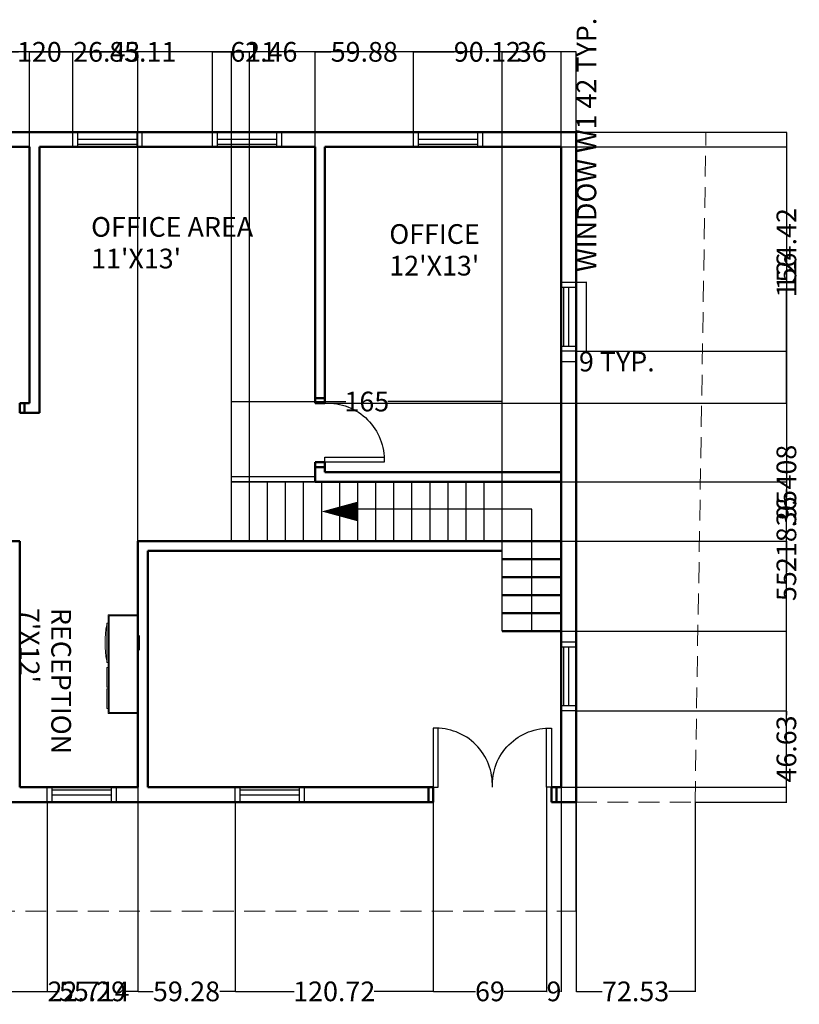
# Model space of a CAD drawing. Units: inches. Extents: x 128 to 1267, y -109 to 1208.
# Tile 8 of 8: x 786 to 1261, y 608 to 1208. Entities that reach past the tile are written whole.
import ezdxf

# ---------------------------------------------------------------- set-up
doc = ezdxf.new("R2010")
doc.units = ezdxf.units.IN
doc.header["$MEASUREMENT"] = 0
doc.linetypes.add('DASHED', pattern=[19.05, 12.7, -6.35])
for name, color, linetype, lineweight in [('A-ANNO-DIMS', 2, 'Continuous', 18), ('A-AREA-IDEN', 3, 'Continuous', 25), ('A-DOOR', 4, 'Continuous', 25), ('A-FLOR-STRS', 2, 'Continuous', 25), ('A-FURN', 8, 'Continuous', 18), ('A-GLAZ', 3, 'Continuous', 25), ('A-ROOF-OVHD', 9, 'DASHED', 18), ('A-WALL', 7, 'Continuous', 50)]:
    doc.layers.add(name, color=color, linetype=linetype, lineweight=lineweight)
doc.styles.get("Standard").update_dxf_attribs({"font": 'arial.ttf'})
doc.dimstyles.get("Standard").update_dxf_attribs({"dimtxt": 12, "dimasz": 0.18, "dimexe": 0.18, "dimexo": 0.0625, "dimgap": 0.09, "dimtad": 0, "dimdec": 1, "dimzin": 0, "dimdsep": 46, "dimlunit": 3, "dimtxsty": 'Standard', "dimcen": 0.09, "dimadec": 0, "dimazin": 0, "dimtfac": 1, "dimtdec": 1, "dimtofl": 0, "dimtmove": 0, "dimatfit": 3, "dimfxl": 1, "dimtolj": 1, "dimtzin": 0, "dimarcsym": 0})

# ---------------------------------------------------------------- blocks, each defined once
blk = doc.blocks.new('Entertainment Center')
for p, q in [((-4, 0), (-5, -1)), ((4, 0), (-4, 0)), ((5, -1), (4, 0)), ((-17, -19), (-17, -1)), ((-17, -1), (43, -1)), ((-16.5, -18.5), (-16.5, -1.5)), ((-16.5, -1.5), (42.5, -1.5)), ((42.5, -1.5), (42.5, -18.5)), ((43, -1), (43, -19)), ((43, -19), (-17, -19)), ((42.5, -18.5), (-16.5, -18.5)), ((-12, -20), (-12, -19)), ((12, -20), (-12, -20)), ((12, -19), (12, -20)), ((15, -20), (15, -19)), ((27, -20), (15, -20)), ((27, -19), (27, -20)), ((28, -20), (28, -19)), ((40, -20), (28, -20)), ((40, -19), (40, -20))]:
    blk.add_line(p, q)
blk.add_arc((0, 40), 61, 259.6111, 280.3889)
blk = doc.blocks.new('DOOR-900')
blk.add_lwpolyline([(460.06, 187.64), (457.06, 187.64), (457.06, 151.64), (460.06, 151.64)], close=True)
blk.add_arc((458.56, 186.14), 34.53, 177.51045, 272.48955)
blk = doc.blocks.new('WIN-900')
for p, q in [((1102.06, 345.56), (1111.06, 345.56)), ((1102.06, 342.56), (1111.06, 342.56)), ((1103.56, 306.56), (1103.56, 342.56)), ((1106.56, 306.56), (1106.56, 342.56)), ((1111.06, 306.56), (1102.06, 306.56)), ((1111.06, 303.56), (1102.06, 303.56))]:
    blk.add_line(p, q)
blk = doc.blocks.new('*D8')
at = {"layer": 'A-ANNO-DIMS', "color": 0, "lineweight": -2, "transparency": 16777216}
for p, q in [((1125.19, 1047.81), (1131.61, 1047.81)), ((1131.43, 1047.81), (1131.43, 1047.99)), ((1131.43, 1005.99), (1131.43, 1047.63)), ((1125.19, 1005.81), (1131.61, 1005.81))]:
    blk.add_line(p, q, dxfattribs=at)
at = {"layer": 'A-ANNO-DIMS', "color": 0, "transparency": 16777216}
for points in [[(1131.4, 1047.63), (1131.46, 1047.63), (1131.43, 1047.81)], [(1131.4, 1005.99), (1131.46, 1005.99), (1131.43, 1005.81)]]:
    blk.add_solid(points, dxfattribs=at)
at = {"layer": 'Defpoints', "color": 0, "transparency": 16777216}
for p in [(1125.13, 1047.81), (1131.43, 1047.81), (1125.13, 1005.81)]:
    blk.add_point(p, dxfattribs=at)
at = {"layer": 'A-ANNO-DIMS', "color": 0, "transparency": 16777216, "insert": (1131.43, 1131.54), "char_height": 12, "attachment_point": 5, "rotation": 90}
blk.add_mtext('\\A1;WINDOW W1 42 TYP.', dxfattribs=at)
blk = doc.blocks.new('*D9')
at = {"layer": 'A-ANNO-DIMS', "color": 0, "lineweight": -2, "transparency": 16777216}
for p, q in [((1116.13, 1005.75), (1116.13, 999.33)), ((1125.13, 1005.75), (1125.13, 999.33)), ((1116.31, 999.51), (1124.95, 999.51)), ((1125.13, 999.51), (1125.31, 999.51))]:
    blk.add_line(p, q, dxfattribs=at)
at = {"layer": 'A-ANNO-DIMS', "color": 0, "transparency": 16777216}
for points in [[(1116.31, 999.54), (1116.31, 999.48), (1116.13, 999.51)], [(1124.95, 999.54), (1124.95, 999.48), (1125.13, 999.51)]]:
    blk.add_solid(points, dxfattribs=at)
at = {"layer": 'Defpoints', "color": 0, "transparency": 16777216}
for p in [(1116.13, 1005.81), (1125.13, 1005.81), (1125.13, 999.51)]:
    blk.add_point(p, dxfattribs=at)
at = {"layer": 'A-ANNO-DIMS', "color": 0, "transparency": 16777216, "insert": (1149.94, 999.51), "char_height": 12, "attachment_point": 5}
blk.add_mtext('\\A1;9 TYP.', dxfattribs=at)
blk = doc.blocks.new('*D93')
at = {"layer": 'A-ANNO-DIMS', "color": 0, "lineweight": -2, "transparency": 16777216}
for p, q in [((237.13, 664.93), (237.13, 1188.36)), ((237.31, 1188.18), (667.76, 1188.18)), ((1124.95, 1188.18), (694.49, 1188.18)), ((1125.13, 664.93), (1125.13, 1188.36))]:
    blk.add_line(p, q, dxfattribs=at)
at = {"layer": 'A-ANNO-DIMS', "color": 0, "transparency": 16777216}
for points in [[(237.31, 1188.21), (237.31, 1188.15), (237.13, 1188.18)], [(1124.95, 1188.21), (1124.95, 1188.15), (1125.13, 1188.18)]]:
    blk.add_solid(points, dxfattribs=at)
at = {"layer": 'Defpoints', "color": 0, "transparency": 16777216}
for p in [(1125.13, 1188.18), (237.13, 664.87), (1125.13, 664.87)]:
    blk.add_point(p, dxfattribs=at)
at = {"layer": 'A-ANNO-DIMS', "color": 0, "transparency": 16777216, "insert": (681.13, 1188.18), "char_height": 12, "attachment_point": 5}
blk.add_mtext('\\A1;888', dxfattribs=at)
blk = doc.blocks.new('*D94')
at = {"layer": 'A-ANNO-DIMS', "color": 0, "lineweight": -2, "transparency": 16777216}
for p, q in [((1125.19, 1139.23), (1253.43, 1139.23)), ((1253.25, 1139.05), (1253.25, 948.83)), ((1253.25, 731.41), (1253.25, 921.63)), ((1197.72, 731.23), (1253.43, 731.23))]:
    blk.add_line(p, q, dxfattribs=at)
at = {"layer": 'A-ANNO-DIMS', "color": 0, "transparency": 16777216}
for points in [[(1253.22, 1139.05), (1253.28, 1139.05), (1253.25, 1139.23)], [(1253.22, 731.41), (1253.28, 731.41), (1253.25, 731.23)]]:
    blk.add_solid(points, dxfattribs=at)
at = {"layer": 'Defpoints', "color": 0, "transparency": 16777216}
for p in [(1125.13, 1139.23), (1197.66, 731.23), (1253.25, 731.23)]:
    blk.add_point(p, dxfattribs=at)
at = {"layer": 'A-ANNO-DIMS', "color": 0, "transparency": 16777216, "insert": (1253.25, 935.23), "char_height": 12, "attachment_point": 5, "rotation": 90}
blk.add_mtext('\\A1;408', dxfattribs=at)
blk = doc.blocks.new('*D95')
at = {"layer": 'A-ANNO-DIMS', "color": 0, "lineweight": -2, "transparency": 16777216}
for p, q in [((1125.13, 731.16), (1125.13, 615.74)), ((1197.66, 731.16), (1197.66, 615.74)), ((1125.31, 615.92), (1141.1, 615.92)), ((1197.48, 615.92), (1181.68, 615.92))]:
    blk.add_line(p, q, dxfattribs=at)
at = {"layer": 'A-ANNO-DIMS', "color": 0, "transparency": 16777216}
for points in [[(1125.31, 615.95), (1125.31, 615.89), (1125.13, 615.92)], [(1197.48, 615.95), (1197.48, 615.89), (1197.66, 615.92)]]:
    blk.add_solid(points, dxfattribs=at)
at = {"layer": 'Defpoints', "color": 0, "transparency": 16777216}
for p in [(1125.13, 731.23), (1197.66, 731.23), (1197.66, 615.92)]:
    blk.add_point(p, dxfattribs=at)
at = {"layer": 'A-ANNO-DIMS', "color": 0, "transparency": 16777216, "insert": (1161.39, 615.92), "char_height": 12, "attachment_point": 5}
blk.add_mtext('\\A1;72.53', dxfattribs=at)
blk = doc.blocks.new('*D106')
at = {"layer": 'A-ANNO-DIMS', "color": 0, "lineweight": -2, "transparency": 16777216}
for p, q in [((708.99, 1139.29), (708.99, 1188.36)), ((709.17, 1188.18), (730.24, 1188.18)), ((791.95, 1188.18), (770.88, 1188.18)), ((792.13, 1130.29), (792.13, 1188.36))]:
    blk.add_line(p, q, dxfattribs=at)
at = {"layer": 'A-ANNO-DIMS', "color": 0, "transparency": 16777216}
for points in [[(709.17, 1188.21), (709.17, 1188.15), (708.99, 1188.18)], [(791.95, 1188.21), (791.95, 1188.15), (792.13, 1188.18)]]:
    blk.add_solid(points, dxfattribs=at)
at = {"layer": 'Defpoints', "color": 0, "transparency": 16777216}
for p in [(792.13, 1188.18), (708.99, 1139.23), (792.13, 1130.23)]:
    blk.add_point(p, dxfattribs=at)
at = {"layer": 'A-ANNO-DIMS', "color": 0, "transparency": 16777216, "insert": (750.56, 1188.18), "char_height": 12, "attachment_point": 5}
blk.add_mtext('\\A1;83.14', dxfattribs=at)
blk = doc.blocks.new('*D107')
at = {"layer": 'A-ANNO-DIMS', "color": 0, "lineweight": -2, "transparency": 16777216}
for p, q in [((792.13, 1130.29), (792.13, 1188.36)), ((792.31, 1188.18), (818.38, 1188.18)), ((818.56, 1139.29), (818.56, 1188.36)), ((818.56, 1188.18), (818.74, 1188.18))]:
    blk.add_line(p, q, dxfattribs=at)
at = {"layer": 'A-ANNO-DIMS', "color": 0, "transparency": 16777216}
for points in [[(792.31, 1188.21), (792.31, 1188.15), (792.13, 1188.18)], [(818.38, 1188.21), (818.38, 1188.15), (818.56, 1188.18)]]:
    blk.add_solid(points, dxfattribs=at)
at = {"layer": 'Defpoints', "color": 0, "transparency": 16777216}
for p in [(818.56, 1188.18), (818.56, 1139.23), (792.13, 1130.23)]:
    blk.add_point(p, dxfattribs=at)
at = {"layer": 'A-ANNO-DIMS', "color": 0, "transparency": 16777216, "insert": (839.18, 1188.18), "char_height": 12, "attachment_point": 5}
blk.add_mtext('\\A1;26.43', dxfattribs=at)
blk = doc.blocks.new('*D108')
at = {"layer": 'A-ANNO-DIMS', "color": 0, "lineweight": -2, "transparency": 16777216}
for p, q in [((818.56, 1139.29), (818.56, 1188.36)), ((818.74, 1188.18), (841.93, 1188.18)), ((903.49, 1188.18), (880.3, 1188.18)), ((903.67, 1139.29), (903.67, 1188.36))]:
    blk.add_line(p, q, dxfattribs=at)
at = {"layer": 'A-ANNO-DIMS', "color": 0, "transparency": 16777216}
for points in [[(818.74, 1188.21), (818.74, 1188.15), (818.56, 1188.18)], [(903.49, 1188.21), (903.49, 1188.15), (903.67, 1188.18)]]:
    blk.add_solid(points, dxfattribs=at)
at = {"layer": 'Defpoints', "color": 0, "transparency": 16777216}
for p in [(903.67, 1188.18), (818.56, 1139.23), (903.67, 1139.23)]:
    blk.add_point(p, dxfattribs=at)
at = {"layer": 'A-ANNO-DIMS', "color": 0, "transparency": 16777216, "insert": (861.11, 1188.18), "char_height": 12, "attachment_point": 5}
blk.add_mtext('\\A1;85.11', dxfattribs=at)
blk = doc.blocks.new('*D109')
at = {"layer": 'A-ANNO-DIMS', "color": 0, "lineweight": -2, "transparency": 16777216}
for p, q in [((903.67, 1139.29), (903.67, 1188.36)), ((903.85, 1188.18), (914.53, 1188.18)), ((965.95, 1188.18), (955.26, 1188.18)), ((966.13, 1130.29), (966.13, 1188.36))]:
    blk.add_line(p, q, dxfattribs=at)
at = {"layer": 'A-ANNO-DIMS', "color": 0, "transparency": 16777216}
for points in [[(903.85, 1188.21), (903.85, 1188.15), (903.67, 1188.18)], [(965.95, 1188.21), (965.95, 1188.15), (966.13, 1188.18)]]:
    blk.add_solid(points, dxfattribs=at)
at = {"layer": 'Defpoints', "color": 0, "transparency": 16777216}
for p in [(966.13, 1188.18), (903.67, 1139.23), (966.13, 1130.23)]:
    blk.add_point(p, dxfattribs=at)
at = {"layer": 'A-ANNO-DIMS', "color": 0, "transparency": 16777216, "insert": (934.9, 1188.18), "char_height": 12, "attachment_point": 5}
blk.add_mtext('\\A1;62.46', dxfattribs=at)
blk = doc.blocks.new('*D110')
at = {"layer": 'A-ANNO-DIMS', "color": 0, "lineweight": -2, "transparency": 16777216}
for p, q in [((966.13, 1130.29), (966.13, 1188.36)), ((966.31, 1188.18), (975.72, 1188.18)), ((1025.83, 1188.18), (1016.42, 1188.18)), ((1026.01, 1139.29), (1026.01, 1188.36))]:
    blk.add_line(p, q, dxfattribs=at)
at = {"layer": 'A-ANNO-DIMS', "color": 0, "transparency": 16777216}
for points in [[(966.31, 1188.21), (966.31, 1188.15), (966.13, 1188.18)], [(1025.83, 1188.21), (1025.83, 1188.15), (1026.01, 1188.18)]]:
    blk.add_solid(points, dxfattribs=at)
at = {"layer": 'Defpoints', "color": 0, "transparency": 16777216}
for p in [(1026.01, 1188.18), (1026.01, 1139.23), (966.13, 1130.23)]:
    blk.add_point(p, dxfattribs=at)
at = {"layer": 'A-ANNO-DIMS', "color": 0, "transparency": 16777216, "insert": (996.07, 1188.18), "char_height": 12, "attachment_point": 5}
blk.add_mtext('\\A1;59.88', dxfattribs=at)
blk = doc.blocks.new('*D111')
at = {"layer": 'A-ANNO-DIMS', "color": 0, "lineweight": -2, "transparency": 16777216}
for p, q in [((1026.01, 1139.29), (1026.01, 1188.36)), ((1026.19, 1188.18), (1050.79, 1188.18)), ((1115.95, 1188.18), (1091.34, 1188.18)), ((1116.13, 1130.29), (1116.13, 1188.36))]:
    blk.add_line(p, q, dxfattribs=at)
at = {"layer": 'A-ANNO-DIMS', "color": 0, "transparency": 16777216}
for points in [[(1026.19, 1188.21), (1026.19, 1188.15), (1026.01, 1188.18)], [(1115.95, 1188.21), (1115.95, 1188.15), (1116.13, 1188.18)]]:
    blk.add_solid(points, dxfattribs=at)
at = {"layer": 'Defpoints', "color": 0, "transparency": 16777216}
for p in [(1116.13, 1188.18), (1026.01, 1139.23), (1116.13, 1130.23)]:
    blk.add_point(p, dxfattribs=at)
at = {"layer": 'A-ANNO-DIMS', "color": 0, "transparency": 16777216, "insert": (1071.07, 1188.18), "char_height": 12, "attachment_point": 5}
blk.add_mtext('\\A1;90.12', dxfattribs=at)
blk = doc.blocks.new('*D120')
at = {"layer": 'A-ANNO-DIMS', "color": 0, "lineweight": -2, "transparency": 16777216}
for p, q in [((780.13, 740.16), (780.13, 615.74)), ((802.84, 731.16), (802.84, 615.74)), ((780.31, 615.92), (802.66, 615.92)), ((802.84, 615.92), (803.02, 615.92))]:
    blk.add_line(p, q, dxfattribs=at)
at = {"layer": 'A-ANNO-DIMS', "color": 0, "transparency": 16777216}
for points in [[(780.31, 615.95), (780.31, 615.89), (780.13, 615.92)], [(802.66, 615.95), (802.66, 615.89), (802.84, 615.92)]]:
    blk.add_solid(points, dxfattribs=at)
at = {"layer": 'Defpoints', "color": 0, "transparency": 16777216}
for p in [(780.13, 740.23), (802.84, 731.23), (802.84, 615.92)]:
    blk.add_point(p, dxfattribs=at)
at = {"layer": 'A-ANNO-DIMS', "color": 0, "transparency": 16777216, "insert": (828.1, 615.92), "char_height": 12, "attachment_point": 5}
blk.add_mtext('\\A1;22.714', dxfattribs=at)
blk = doc.blocks.new('*D121')
at = {"layer": 'A-ANNO-DIMS', "color": 0, "lineweight": -2, "transparency": 16777216}
for p, q in [((858.13, 740.16), (858.13, 615.74)), ((802.84, 731.16), (802.84, 615.74)), ((803.02, 615.92), (810.13, 615.92)), ((857.95, 615.92), (850.83, 615.92))]:
    blk.add_line(p, q, dxfattribs=at)
at = {"layer": 'A-ANNO-DIMS', "color": 0, "transparency": 16777216}
for points in [[(803.02, 615.95), (803.02, 615.89), (802.84, 615.92)], [(857.95, 615.95), (857.95, 615.89), (858.13, 615.92)]]:
    blk.add_solid(points, dxfattribs=at)
at = {"layer": 'Defpoints', "color": 0, "transparency": 16777216}
for p in [(858.13, 740.23), (802.84, 731.23), (858.13, 615.92)]:
    blk.add_point(p, dxfattribs=at)
at = {"layer": 'A-ANNO-DIMS', "color": 0, "transparency": 16777216, "insert": (830.48, 615.92), "char_height": 12, "attachment_point": 5}
blk.add_mtext('\\A1;55.29', dxfattribs=at)
blk = doc.blocks.new('*D122')
at = {"layer": 'A-ANNO-DIMS', "color": 0, "lineweight": -2, "transparency": 16777216}
for p, q in [((858.13, 740.16), (858.13, 615.74)), ((917.41, 731.16), (917.41, 615.74)), ((858.31, 615.92), (867.42, 615.92)), ((917.23, 615.92), (908.12, 615.92))]:
    blk.add_line(p, q, dxfattribs=at)
at = {"layer": 'A-ANNO-DIMS', "color": 0, "transparency": 16777216}
for points in [[(858.31, 615.95), (858.31, 615.89), (858.13, 615.92)], [(917.23, 615.95), (917.23, 615.89), (917.41, 615.92)]]:
    blk.add_solid(points, dxfattribs=at)
at = {"layer": 'Defpoints', "color": 0, "transparency": 16777216}
for p in [(858.13, 740.23), (917.41, 731.23), (917.41, 615.92)]:
    blk.add_point(p, dxfattribs=at)
at = {"layer": 'A-ANNO-DIMS', "color": 0, "transparency": 16777216, "insert": (887.77, 615.92), "char_height": 12, "attachment_point": 5}
blk.add_mtext('\\A1;59.28', dxfattribs=at)
blk = doc.blocks.new('*D123')
at = {"layer": 'A-ANNO-DIMS', "color": 0, "lineweight": -2, "transparency": 16777216}
for p, q in [((917.41, 731.16), (917.41, 615.74)), ((1038.13, 731.16), (1038.13, 615.74)), ((917.59, 615.92), (953.4, 615.92)), ((1037.95, 615.92), (1002.14, 615.92))]:
    blk.add_line(p, q, dxfattribs=at)
at = {"layer": 'A-ANNO-DIMS', "color": 0, "transparency": 16777216}
for points in [[(917.59, 615.95), (917.59, 615.89), (917.41, 615.92)], [(1037.95, 615.95), (1037.95, 615.89), (1038.13, 615.92)]]:
    blk.add_solid(points, dxfattribs=at)
at = {"layer": 'Defpoints', "color": 0, "transparency": 16777216}
for p in [(917.41, 731.23), (1038.13, 731.23), (1038.13, 615.92)]:
    blk.add_point(p, dxfattribs=at)
at = {"layer": 'A-ANNO-DIMS', "color": 0, "transparency": 16777216, "insert": (977.77, 615.92), "char_height": 12, "attachment_point": 5}
blk.add_mtext('\\A1;120.72', dxfattribs=at)
blk = doc.blocks.new('*D124')
at = {"layer": 'A-ANNO-DIMS', "color": 0, "lineweight": -2, "transparency": 16777216}
for p, q in [((1107.13, 740.16), (1107.13, 615.74)), ((1038.13, 731.16), (1038.13, 615.74)), ((1038.31, 615.92), (1063.9, 615.92)), ((1106.95, 615.92), (1081.36, 615.92))]:
    blk.add_line(p, q, dxfattribs=at)
at = {"layer": 'A-ANNO-DIMS', "color": 0, "transparency": 16777216}
for points in [[(1038.31, 615.95), (1038.31, 615.89), (1038.13, 615.92)], [(1106.95, 615.95), (1106.95, 615.89), (1107.13, 615.92)]]:
    blk.add_solid(points, dxfattribs=at)
at = {"layer": 'Defpoints', "color": 0, "transparency": 16777216}
for p in [(1107.13, 740.23), (1038.13, 731.23), (1107.13, 615.92)]:
    blk.add_point(p, dxfattribs=at)
at = {"layer": 'A-ANNO-DIMS', "color": 0, "transparency": 16777216, "insert": (1072.63, 615.92), "char_height": 12, "attachment_point": 5}
blk.add_mtext('\\A1;69', dxfattribs=at)
blk = doc.blocks.new('*D125')
at = {"layer": 'A-ANNO-DIMS', "color": 0, "lineweight": -2, "transparency": 16777216}
for p, q in [((1107.13, 740.16), (1107.13, 615.74)), ((1116.13, 740.16), (1116.13, 615.74)), ((1107.31, 615.92), (1107.59, 615.92)), ((1115.95, 615.92), (1115.66, 615.92))]:
    blk.add_line(p, q, dxfattribs=at)
at = {"layer": 'A-ANNO-DIMS', "color": 0, "transparency": 16777216}
for points in [[(1107.31, 615.95), (1107.31, 615.89), (1107.13, 615.92)], [(1115.95, 615.95), (1115.95, 615.89), (1116.13, 615.92)]]:
    blk.add_solid(points, dxfattribs=at)
at = {"layer": 'Defpoints', "color": 0, "transparency": 16777216}
for p in [(1107.13, 740.23), (1116.13, 740.23), (1116.13, 615.92)]:
    blk.add_point(p, dxfattribs=at)
at = {"layer": 'A-ANNO-DIMS', "color": 0, "transparency": 16777216, "insert": (1111.63, 615.92), "char_height": 12, "attachment_point": 5}
blk.add_mtext('\\A1;9', dxfattribs=at)
blk = doc.blocks.new('*D130')
at = {"layer": 'A-ANNO-DIMS', "color": 0, "lineweight": -2, "transparency": 16777216}
for p, q in [((1125.19, 786.85), (1253.43, 786.85)), ((1253.25, 786.67), (1253.25, 784.12)), ((1116.19, 740.23), (1253.43, 740.23)), ((1253.25, 740.41), (1253.25, 742.96))]:
    blk.add_line(p, q, dxfattribs=at)
at = {"layer": 'A-ANNO-DIMS', "color": 0, "transparency": 16777216}
for points in [[(1253.22, 786.67), (1253.28, 786.67), (1253.25, 786.85)], [(1253.22, 740.41), (1253.28, 740.41), (1253.25, 740.23)]]:
    blk.add_solid(points, dxfattribs=at)
at = {"layer": 'Defpoints', "color": 0, "transparency": 16777216}
for p in [(1125.13, 786.85), (1253.25, 786.85), (1116.13, 740.23)]:
    blk.add_point(p, dxfattribs=at)
at = {"layer": 'A-ANNO-DIMS', "color": 0, "transparency": 16777216, "insert": (1253.25, 763.54), "char_height": 12, "attachment_point": 5, "rotation": 90}
blk.add_mtext('\\A1;46.63', dxfattribs=at)
blk = doc.blocks.new('*D131')
at = {"layer": 'A-ANNO-DIMS', "color": 0, "lineweight": -2, "transparency": 16777216}
for p, q in [((1125.19, 1005.81), (1253.43, 1005.81)), ((1253.25, 1005.63), (1253.25, 921.48)), ((1253.25, 787.03), (1253.25, 871.19)), ((1125.19, 786.85), (1253.43, 786.85))]:
    blk.add_line(p, q, dxfattribs=at)
at = {"layer": 'A-ANNO-DIMS', "color": 0, "transparency": 16777216}
for points in [[(1253.22, 1005.63), (1253.28, 1005.63), (1253.25, 1005.81)], [(1253.22, 787.03), (1253.28, 787.03), (1253.25, 786.85)]]:
    blk.add_solid(points, dxfattribs=at)
at = {"layer": 'Defpoints', "color": 0, "transparency": 16777216}
for p in [(1125.13, 1005.81), (1253.25, 1005.81), (1125.13, 786.85)]:
    blk.add_point(p, dxfattribs=at)
at = {"layer": 'A-ANNO-DIMS', "color": 0, "transparency": 16777216, "insert": (1253.25, 896.33), "char_height": 12, "attachment_point": 5, "rotation": 90}
blk.add_mtext('\\A1;218.95', dxfattribs=at)
blk = doc.blocks.new('*D132')
at = {"layer": 'A-ANNO-DIMS', "color": 0, "lineweight": -2, "transparency": 16777216}
for p, q in [((1116.19, 1130.23), (1253.43, 1130.23)), ((1253.25, 1130.05), (1253.25, 1092.39)), ((1253.25, 1005.99), (1253.25, 1043.64)), ((1125.19, 1005.81), (1253.43, 1005.81))]:
    blk.add_line(p, q, dxfattribs=at)
at = {"layer": 'A-ANNO-DIMS', "color": 0, "transparency": 16777216}
for points in [[(1253.22, 1130.05), (1253.28, 1130.05), (1253.25, 1130.23)], [(1253.22, 1005.99), (1253.28, 1005.99), (1253.25, 1005.81)]]:
    blk.add_solid(points, dxfattribs=at)
at = {"layer": 'Defpoints', "color": 0, "transparency": 16777216}
for p in [(1116.13, 1130.23), (1253.25, 1130.23), (1125.13, 1005.81)]:
    blk.add_point(p, dxfattribs=at)
at = {"layer": 'A-ANNO-DIMS', "color": 0, "transparency": 16777216, "insert": (1253.25, 1068.02), "char_height": 12, "attachment_point": 5, "rotation": 90}
blk.add_mtext('\\A1;124.42', dxfattribs=at)
blk = doc.blocks.new('*D133')
at = {"layer": 'A-ANNO-DIMS', "color": 0, "lineweight": -2, "transparency": 16777216}
for p, q in [((1080.19, 890.23), (1253.43, 890.23)), ((1253.25, 890.05), (1253.25, 871.46)), ((1253.25, 835.41), (1253.25, 854)), ((1080.19, 835.23), (1253.43, 835.23))]:
    blk.add_line(p, q, dxfattribs=at)
at = {"layer": 'A-ANNO-DIMS', "color": 0, "transparency": 16777216}
for points in [[(1253.22, 890.05), (1253.28, 890.05), (1253.25, 890.23)], [(1253.22, 835.41), (1253.28, 835.41), (1253.25, 835.23)]]:
    blk.add_solid(points, dxfattribs=at)
at = {"layer": 'Defpoints', "color": 0, "transparency": 16777216}
for p in [(1080.13, 890.23), (1080.13, 835.23), (1253.25, 835.23)]:
    blk.add_point(p, dxfattribs=at)
at = {"layer": 'A-ANNO-DIMS', "color": 0, "transparency": 16777216, "insert": (1253.25, 862.73), "char_height": 12, "attachment_point": 5, "rotation": 90}
blk.add_mtext('\\A1;55', dxfattribs=at)
blk = doc.blocks.new('*D142')
at = {"layer": 'A-ANNO-DIMS', "color": 0, "lineweight": -2, "transparency": 16777216}
for p, q in [((915.13, 926.29), (915.13, 975.36)), ((915.31, 975.18), (984.8, 975.18)), ((1079.95, 975.18), (1010.45, 975.18)), ((1080.13, 926.29), (1080.13, 975.36))]:
    blk.add_line(p, q, dxfattribs=at)
at = {"layer": 'A-ANNO-DIMS', "color": 0, "transparency": 16777216}
for points in [[(915.31, 975.21), (915.31, 975.15), (915.13, 975.18)], [(1079.95, 975.21), (1079.95, 975.15), (1080.13, 975.18)]]:
    blk.add_solid(points, dxfattribs=at)
at = {"layer": 'Defpoints', "color": 0, "transparency": 16777216}
for p in [(1080.13, 975.18), (915.13, 926.23), (1080.13, 926.23)]:
    blk.add_point(p, dxfattribs=at)
at = {"layer": 'A-ANNO-DIMS', "color": 0, "transparency": 16777216, "insert": (997.63, 975.18), "char_height": 12, "attachment_point": 5}
blk.add_mtext('\\A1;165', dxfattribs=at)
blk = doc.blocks.new('*D143')
at = {"layer": 'A-ANNO-DIMS', "color": 0, "lineweight": -2, "transparency": 16777216}
for p, q in [((915.19, 926.23), (1253.43, 926.23)), ((1253.25, 926.05), (1253.25, 916.9)), ((1253.25, 890.41), (1253.25, 899.55)), ((915.19, 890.23), (1253.43, 890.23))]:
    blk.add_line(p, q, dxfattribs=at)
at = {"layer": 'A-ANNO-DIMS', "color": 0, "transparency": 16777216}
for points in [[(1253.22, 926.05), (1253.28, 926.05), (1253.25, 926.23)], [(1253.22, 890.41), (1253.28, 890.41), (1253.25, 890.23)]]:
    blk.add_solid(points, dxfattribs=at)
at = {"layer": 'Defpoints', "color": 0, "transparency": 16777216}
for p in [(915.13, 926.23), (915.13, 890.23), (1253.25, 890.23)]:
    blk.add_point(p, dxfattribs=at)
at = {"layer": 'A-ANNO-DIMS', "color": 0, "transparency": 16777216, "insert": (1253.25, 908.23), "char_height": 12, "attachment_point": 5, "rotation": 90}
blk.add_mtext('\\A1;36', dxfattribs=at)
blk = doc.blocks.new('*D144')
at = {"layer": 'A-ANNO-DIMS', "color": 0, "lineweight": -2, "transparency": 16777216}
for p, q in [((915.13, 926.29), (915.13, 1188.36)), ((915.31, 1188.18), (925.95, 1188.18)), ((926.13, 926.29), (926.13, 1188.36)), ((926.13, 1188.18), (926.31, 1188.18))]:
    blk.add_line(p, q, dxfattribs=at)
at = {"layer": 'A-ANNO-DIMS', "color": 0, "transparency": 16777216}
for points in [[(915.31, 1188.21), (915.31, 1188.15), (915.13, 1188.18)], [(925.95, 1188.21), (925.95, 1188.15), (926.13, 1188.18)]]:
    blk.add_solid(points, dxfattribs=at)
at = {"layer": 'Defpoints', "color": 0, "transparency": 16777216}
for p in [(926.13, 1188.18), (915.13, 926.23), (926.13, 926.23)]:
    blk.add_point(p, dxfattribs=at)
at = {"layer": 'A-ANNO-DIMS', "color": 0, "transparency": 16777216, "insert": (933.27, 1188.18), "char_height": 12, "attachment_point": 5}
blk.add_mtext('\\A1;11', dxfattribs=at)
blk = doc.blocks.new('*D145')
at = {"layer": 'A-ANNO-DIMS', "color": 0, "lineweight": -2, "transparency": 16777216}
for p, q in [((1080.13, 926.29), (1080.13, 1188.36)), ((1080.31, 1188.18), (1089.45, 1188.18)), ((1115.95, 1188.18), (1106.8, 1188.18)), ((1116.13, 926.29), (1116.13, 1188.36))]:
    blk.add_line(p, q, dxfattribs=at)
at = {"layer": 'A-ANNO-DIMS', "color": 0, "transparency": 16777216}
for points in [[(1080.31, 1188.21), (1080.31, 1188.15), (1080.13, 1188.18)], [(1115.95, 1188.21), (1115.95, 1188.15), (1116.13, 1188.18)]]:
    blk.add_solid(points, dxfattribs=at)
at = {"layer": 'Defpoints', "color": 0, "transparency": 16777216}
for p in [(1116.13, 1188.18), (1080.13, 926.23), (1116.13, 926.23)]:
    blk.add_point(p, dxfattribs=at)
at = {"layer": 'A-ANNO-DIMS', "color": 0, "transparency": 16777216, "insert": (1098.13, 1188.18), "char_height": 12, "attachment_point": 5}
blk.add_mtext('\\A1;36', dxfattribs=at)
blk = doc.blocks.new('*D146')
at = {"layer": 'A-ANNO-DIMS', "color": 0, "lineweight": -2, "transparency": 16777216}
for p, q in [((972.19, 1130.23), (1253.43, 1130.23)), ((1253.25, 1130.05), (1253.25, 1065)), ((1253.25, 974.41), (1253.25, 1039.45)), ((972.19, 974.23), (1253.43, 974.23))]:
    blk.add_line(p, q, dxfattribs=at)
at = {"layer": 'A-ANNO-DIMS', "color": 0, "transparency": 16777216}
for points in [[(1253.22, 1130.05), (1253.28, 1130.05), (1253.25, 1130.23)], [(1253.22, 974.41), (1253.28, 974.41), (1253.25, 974.23)]]:
    blk.add_solid(points, dxfattribs=at)
at = {"layer": 'Defpoints', "color": 0, "transparency": 16777216}
for p in [(972.13, 1130.23), (1253.25, 1130.23), (972.13, 974.23)]:
    blk.add_point(p, dxfattribs=at)
at = {"layer": 'A-ANNO-DIMS', "color": 0, "transparency": 16777216, "insert": (1253.25, 1052.23), "char_height": 12, "attachment_point": 5, "rotation": 90}
blk.add_mtext('\\A1;156', dxfattribs=at)
blk = doc.blocks.new('*D155')
at = {"layer": 'A-ANNO-DIMS', "color": 0, "lineweight": -2, "transparency": 16777216}
for p, q in [((738.13, 890.29), (738.13, 1188.36)), ((738.31, 1188.18), (785.37, 1188.18)), ((857.95, 1188.18), (810.89, 1188.18)), ((858.13, 890.29), (858.13, 1188.36))]:
    blk.add_line(p, q, dxfattribs=at)
at = {"layer": 'A-ANNO-DIMS', "color": 0, "transparency": 16777216}
for points in [[(738.31, 1188.21), (738.31, 1188.15), (738.13, 1188.18)], [(857.95, 1188.21), (857.95, 1188.15), (858.13, 1188.18)]]:
    blk.add_solid(points, dxfattribs=at)
at = {"layer": 'Defpoints', "color": 0, "transparency": 16777216}
for p in [(858.13, 1188.18), (738.13, 890.23), (858.13, 890.23)]:
    blk.add_point(p, dxfattribs=at)
at = {"layer": 'A-ANNO-DIMS', "color": 0, "transparency": 16777216, "insert": (798.13, 1188.18), "char_height": 12, "attachment_point": 5}
blk.add_mtext('\\A1;120', dxfattribs=at)

msp = doc.modelspace()

# ---------------------------------------------------------------- linework, layer by layer
at = {"layer": 'A-FLOR-STRS'}
for p, q in [((966.1268, 929.2265), (915.1268, 929.2265)), ((915.1268, 926.2265), (915.1268, 929.2265)), ((966.1268, 926.2265), (915.1268, 926.2265)), ((915.1268, 890.2265), (915.1268, 926.2265)), ((926.1268, 890.2265), (926.1268, 926.2265)), ((937.1268, 890.2265), (937.1268, 926.2265)), ((948.1268, 890.2265), (948.1268, 926.2265)), ((959.1268, 890.2265), (959.1268, 926.2265)), ((970.1268, 890.2265), (970.1268, 926.2265)), ((981.1268, 890.2265), (981.1268, 926.2265)), ((992.1268, 890.2265), (992.1268, 926.2265)), ((1003.1268, 890.2265), (1003.1268, 926.2265)), ((1014.1268, 890.2265), (1014.1268, 926.2265)), ((1025.1268, 890.2265), (1025.1268, 926.2265)), ((1036.1268, 890.2265), (1036.1268, 926.2265)), ((1047.1268, 890.2265), (1047.1268, 926.2265)), ((1058.1268, 890.2265), (1058.1268, 926.2265)), ((1069.1268, 890.2265), (1069.1268, 926.2265)), ((1080.1268, 890.2265), (1080.1268, 926.2265)), ((1080.1268, 835.2265), (1080.1268, 890.2265))]:
    msp.add_line(p, q, dxfattribs=at)
msp.add_lwpolyline([(992.1268, 908.2265, 12, 0, 0), (970.1268, 908.2265, 0, 0, 0)], format="xyseb", dxfattribs=at)
msp.add_lwpolyline([(1098.1268, 835.2265), (1098.1268, 909.6587), (992.1268, 909.6587)], dxfattribs=at)
at = {"layer": 'A-ROOF-OVHD'}
for p, q in [((1125.1268, 1139.2265), (1204.3015, 1139.2265)), ((1197.658, 731.2265), (1204.2378, 1139.2265)), ((1125.1268, 731.2265), (1125.1268, 664.8687)), ((1125.1268, 731.2265), (1197.658, 731.2265)), ((237.1268, 664.8687), (1125.1268, 664.8687))]:
    msp.add_line(p, q, dxfattribs=at)
at = {"layer": 'A-WALL'}
for p, q in [((792.1268, 1130.2265), (672.1268, 1130.2265)), ((792.1268, 974.2265), (792.1268, 1130.2265)), ((798.1268, 968.2265), (798.1268, 1130.2265)), ((966.1268, 1130.2265), (798.1268, 1130.2265)), ((966.1268, 974.2265), (966.1268, 1130.2265)), ((1116.1268, 1130.2265), (972.1268, 1130.2265)), ((972.1268, 974.2265), (972.1268, 1130.2265)), ((1116.1268, 974.2265), (1116.1268, 1130.2265)), ((1116.1268, 932.2265), (1116.1268, 1130.2265)), ((792.1268, 974.2265), (786.1268, 974.2265)), ((786.1268, 974.2265), (786.1268, 968.2265)), ((789.1268, 974.2265), (789.1268, 968.2265)), ((972.1268, 977.2265), (966.1268, 977.2265)), ((972.1268, 974.2265), (966.1268, 974.2265)), ((798.1268, 968.2265), (786.1268, 968.2265)), ((1116.1268, 890.2265), (1116.1268, 968.2265)), ((1116.1268, 890.2265), (1116.1268, 968.2265)), ((966.1268, 926.2265), (966.1268, 938.2265)), ((972.1268, 938.2265), (966.1268, 938.2265)), ((972.1268, 932.2265), (972.1268, 938.2265)), ((972.1268, 935.2265), (966.1268, 935.2265)), ((972.1268, 932.2265), (1116.1268, 932.2265)), ((966.1268, 926.2265), (1116.1268, 926.2265)), ((774.1268, 890.2265), (786.1268, 890.2265)), ((786.1268, 890.2265), (786.1268, 740.2265)), ((858.1268, 890.2265), (858.1268, 740.2265)), ((858.1268, 890.2265), (1080.1268, 890.2265)), ((1080.1268, 890.2265), (1116.1268, 890.2265)), ((1116.1268, 740.2265), (1116.1268, 890.2265)), ((864.1268, 884.2265), (1080.1268, 884.2265)), ((864.1268, 884.2265), (864.1268, 740.2265)), ((1080.1268, 879.2265), (1116.1268, 879.2265)), ((1080.1268, 868.2265), (1116.1268, 868.2265)), ((1080.1268, 857.2265), (1116.1268, 857.2265)), ((1080.1268, 846.2265), (1116.1268, 846.2265)), ((1080.1268, 835.2265), (1116.1268, 835.2265)), ((786.1268, 740.2265), (858.1268, 740.2265)), ((864.1268, 740.2265), (1038.1268, 740.2265)), ((1035.1268, 740.2265), (1035.1268, 731.2265)), ((1038.1268, 740.2265), (1038.1268, 731.2265)), ((1110.1268, 740.2265), (1110.1268, 731.2265)), ((1110.1268, 740.2265), (1116.1268, 740.2265)), ((1113.1268, 740.2265), (1113.1268, 731.2265))]:
    msp.add_line(p, q, dxfattribs=at)
msp.add_lwpolyline([(1110.1268, 731.2265), (1125.1268, 731.2265), (1125.1268, 1139.2265), (237.1268, 1139.2265), (237.1268, 731.2265), (1038.1268, 731.2265)], dxfattribs=at)

# ---------------------------------------------------------------- block references
at = {"layer": 'A-DOOR', "extrusion": (0, 0, -1), "zscale": -1}
for p, rotation in [((-1159.7667, 1398.2825), 270.0000000000002), ((-650.0707, 927.8664), 180)]:
    msp.add_blockref('DOOR-900', p, dxfattribs=dict(at, rotation=rotation))
at = {"layer": 'A-DOOR', "rotation": 180}
msp.add_blockref('DOOR-900', (1498.1828, 927.8664), dxfattribs=at)
at = {"layer": 'A-FURN', "rotation": 269.9999999999477}
msp.add_blockref('Entertainment Center', (859.1268, 828.2265), dxfattribs=at)
at = {"layer": 'A-GLAZ'}
for p, rotation in [((1164.1183, 28.1705), 90.00000000000104), ((1249.2326, 28.1705), 90.00000000000104), ((1371.569, 28.1705), 90.0000000000011), ((499.2788, 1842.2825), 270.0000000000003), ((613.8478, 1842.2825), 270.0000000000003)]:
    msp.add_blockref('WIN-900', p, dxfattribs=dict(at, rotation=rotation))
for p in [(14.0707, 702.2454), (14.0707, 483.2925)]:
    msp.add_blockref('WIN-900', p, dxfattribs=at)

# ---------------------------------------------------------------- texts
at = {"layer": 'A-AREA-IDEN'}
for s, p in [('OFFICE AREA', (829.6489, 1075.5634)), ('OFFICE', (1011.3284, 1071.2173)), ("11'X13'", (829.6489, 1056.2864)), ("12'X13'", (1011.3284, 1051.9404))]:
    msp.add_text(s, height=12, dxfattribs=at).set_placement(p)
for s, p in [("7'X12'", (786.1268, 849.489)), ('RECEPTION', (805.4037, 849.489))]:
    msp.add_text(s, height=12, rotation=270, dxfattribs=at).set_placement(p)

# ---------------------------------------------------------------- dimensions: what is measured, and where the dimension line sits
at = {"layer": 'A-ANNO-DIMS'}
dim = msp.add_linear_dim(base=(1131.4268, 1047.8077), p1=(1125.1268, 1005.8077), p2=(1125.1268, 1047.8077), angle=90, text='WINDOW W1 <> TYP.', dimstyle='Standard', override={"dimdec": 0, "dimrnd": 0, "dimzin": 0, "dimlunit": 2}, dxfattribs=at)
dim.commit()
dim.dimension.update_dxf_attribs({"geometry": '*D8', "text_midpoint": (1131.4268, 1131.5375)})
for base, p1, p2, override, picture, middle in [((1125.1268, 1188.1765), (237.1268, 664.8687), (1125.1268, 664.8687), {"dimdec": 0, "dimlfac": 1, "dimrnd": 0, "dimzin": 0, "dimdsep": 46, "dimlunit": 2}, '*D93', (681.1268, 1188.1765)), ((792.1268, 1188.1765), (708.9852, 1139.2265), (792.1268, 1130.2265), {"dimdec": 2, "dimlfac": 1, "dimrnd": 0, "dimzin": 0, "dimdsep": 46, "dimlunit": 2}, '*D106', (750.556, 1188.1765)), ((858.1268, 1188.1765), (738.1268, 890.2265), (858.1268, 890.2265), {"dimdec": 0, "dimlfac": 1, "dimrnd": 0, "dimzin": 0, "dimdsep": 46, "dimlunit": 2}, '*D155', (798.1268, 1188.1765)), ((818.556, 1188.1765), (792.1268, 1130.2265), (818.556, 1139.2265), {"dimdec": 2, "dimlfac": 1, "dimrnd": 0, "dimzin": 0, "dimdsep": 46, "dimlunit": 2}, '*D107', (839.1753, 1188.1765)), ((903.6703, 1188.1765), (818.556, 1139.2265), (903.6703, 1139.2265), {"dimdec": 2, "dimlfac": 1, "dimrnd": 0, "dimzin": 0, "dimdsep": 46, "dimlunit": 2}, '*D108', (861.1132, 1188.1765)), ((966.1268, 1188.1765), (903.6703, 1139.2265), (966.1268, 1130.2265), {"dimdec": 2, "dimlfac": 1, "dimrnd": 0, "dimzin": 0, "dimdsep": 46, "dimlunit": 2}, '*D109', (934.8985, 1188.1765)), ((926.1268, 1188.1765), (915.1268, 926.2265), (926.1268, 926.2265), {"dimdec": 0, "dimlfac": 1, "dimrnd": 0, "dimzin": 0, "dimdsep": 46, "dimlunit": 2}, '*D144', (933.2685, 1188.1765)), ((1026.0067, 1188.1765), (966.1268, 1130.2265), (1026.0067, 1139.2265), {"dimdec": 2, "dimlfac": 1, "dimrnd": 0, "dimzin": 0, "dimdsep": 46, "dimlunit": 2}, '*D110', (996.0667, 1188.1765)), ((1116.1268, 1188.1765), (1026.0067, 1139.2265), (1116.1268, 1130.2265), {"dimdec": 2, "dimlfac": 1, "dimrnd": 0, "dimzin": 0, "dimdsep": 46, "dimlunit": 2}, '*D111', (1071.0667, 1188.1765)), ((1116.1268, 1188.1765), (1080.1268, 926.2265), (1116.1268, 926.2265), {"dimdec": 0, "dimlfac": 1, "dimrnd": 0, "dimzin": 0, "dimdsep": 46, "dimlunit": 2}, '*D145', (1098.1268, 1188.1765)), ((802.8411, 615.9187), (780.1268, 740.2265), (802.8411, 731.2265), {"dimdec": 3, "dimlfac": 1, "dimrnd": 0, "dimzin": 0, "dimdsep": 46, "dimlunit": 2}, '*D120', (828.0975, 615.9187)), ((858.1268, 615.9187), (802.8411, 731.2265), (858.1268, 740.2265), {"dimdec": 2, "dimlfac": 1, "dimrnd": 0, "dimzin": 0, "dimdsep": 46, "dimlunit": 2}, '*D121', (830.4839, 615.9187)), ((917.4101, 615.9187), (858.1268, 740.2265), (917.4101, 731.2265), {"dimdec": 2, "dimlfac": 1, "dimrnd": 0, "dimzin": 0, "dimdsep": 46, "dimlunit": 2}, '*D122', (887.7685, 615.9187)), ((1107.1268, 615.9187), (1038.1268, 731.2265), (1107.1268, 740.2265), {"dimdec": 0, "dimlfac": 1, "dimrnd": 0, "dimzin": 0, "dimdsep": 46, "dimlunit": 2}, '*D124', (1072.6268, 615.9187)), ((1116.1268, 615.9187), (1107.1268, 740.2265), (1116.1268, 740.2265), {"dimdec": 0, "dimlfac": 1, "dimrnd": 0, "dimzin": 0, "dimdsep": 46, "dimlunit": 2}, '*D125', (1111.6268, 615.9187)), ((1038.1268, 615.9187), (917.4101, 731.2265), (1038.1268, 731.2265), {"dimdec": 2, "dimlfac": 1, "dimrnd": 0, "dimzin": 0, "dimdsep": 46, "dimlunit": 2}, '*D123', (977.7685, 615.9187)), ((1197.658, 615.9187), (1125.1268, 731.2265), (1197.658, 731.2265), {"dimdec": 2, "dimlfac": 1, "dimrnd": 0, "dimzin": 0, "dimdsep": 46, "dimlunit": 2}, '*D95', (1161.3924, 615.9187))]:
    dim = msp.add_linear_dim(base=base, p1=p1, p2=p2, dimstyle='Standard', override=override, dxfattribs=at)
    dim.commit()
    dim.dimension.update_dxf_attribs({"geometry": picture, "text_midpoint": middle})
for base, p1, p2, angle, override, picture, middle in [((1253.2515, 731.2265), (1125.1268, 1139.2265), (1197.658, 731.2265), 90, {"dimdec": 0, "dimlfac": 1, "dimrnd": 0, "dimzin": 0, "dimdsep": 46, "dimlunit": 2}, '*D94', (1253.2515, 935.2265)), ((1253.2515, 1130.2265), (972.1268, 974.2265), (972.1268, 1130.2265), 90, {"dimdec": 0, "dimlfac": 1, "dimrnd": 0, "dimzin": 0, "dimdsep": 46, "dimlunit": 2}, '*D146', (1253.2515, 1052.2265)), ((1253.2515, 1130.2265), (1125.1268, 1005.8077), (1116.1268, 1130.2265), 90, {"dimdec": 2, "dimlfac": 1, "dimrnd": 0, "dimzin": 0, "dimdsep": 46, "dimlunit": 2}, '*D132', (1253.2515, 1068.0171)), ((1253.2515, 1005.8077), (1125.1268, 786.8549), (1125.1268, 1005.8077), 90, {"dimdec": 2, "dimlfac": 1, "dimrnd": 0, "dimzin": 0, "dimdsep": 46, "dimlunit": 2}, '*D131', (1253.2515, 896.3313)), ((1080.1268, 975.1765), (915.1268, 926.2265), (1080.1268, 926.2265), 0, {"dimdec": 0, "dimlfac": 1, "dimrnd": 0, "dimzin": 0, "dimdsep": 46, "dimlunit": 2}, '*D142', (997.6268, 975.1765)), ((1253.2515, 890.2265), (915.1268, 926.2265), (915.1268, 890.2265), 90, {"dimdec": 0, "dimlfac": 1, "dimrnd": 0, "dimzin": 0, "dimdsep": 46, "dimlunit": 2}, '*D143', (1253.2515, 908.2265)), ((1253.2515, 835.2265), (1080.1268, 890.2265), (1080.1268, 835.2265), 90, {"dimdec": 0, "dimlfac": 1, "dimrnd": 0, "dimzin": 0, "dimdsep": 46, "dimlunit": 2}, '*D133', (1253.2515, 862.7265)), ((1253.2515, 786.8549), (1116.1268, 740.2265), (1125.1268, 786.8549), 90, {"dimdec": 2, "dimlfac": 1, "dimrnd": 0, "dimzin": 0, "dimdsep": 46, "dimlunit": 2}, '*D130', (1253.2515, 763.5407))]:
    dim = msp.add_linear_dim(base=base, p1=p1, p2=p2, angle=angle, dimstyle='Standard', override=override, dxfattribs=at)
    dim.commit()
    dim.dimension.update_dxf_attribs({"geometry": picture, "text_midpoint": middle})
dim = msp.add_linear_dim(base=(1125.1268, 999.5077), p1=(1116.1268, 1005.8077), p2=(1125.1268, 1005.8077), text='<> TYP.', dimstyle='Standard', override={"dimdec": 0, "dimrnd": 0, "dimzin": 0, "dimlunit": 2}, dxfattribs=at)
dim.commit()
dim.dimension.update_dxf_attribs({"geometry": '*D9', "text_midpoint": (1149.9411, 999.5077)})

doc.saveas('drawing.dxf')
